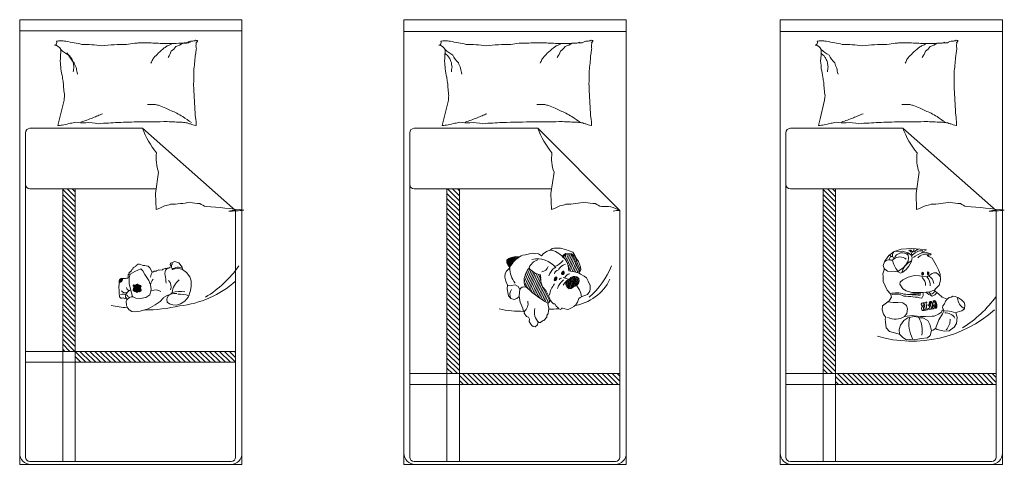
# Model space of a CAD drawing. Units: inches. Extents: x -17 to 1735, y -531 to 60.
# Tile 5 of 27: x 1734.6625 to 1734.8369, y -150.3996 to -150.3208. Entities that reach past the tile are written whole.
import ezdxf

# ---------------------------------------------------------------- set-up
doc = ezdxf.new("R2010")
doc.units = ezdxf.units.IN
doc.header["$MEASUREMENT"] = 0
doc.layers.add('A-FURN', color=242, linetype='Continuous', lineweight=18, true_color=0xcd2027)
pattern_1 = [(45, (81.6226725, 61.5392477), (-0.0019250982, 0.0019250982), [])]

# ---------------------------------------------------------------- blocks, each defined once
blk = doc.blocks.new('childrens_room_2')
h = blk.add_hatch()
h.set_pattern_fill('ANSI31', color=256, scale=0.005, style=0)
h.set_pattern_definition([(135, (71.032121, 52.193135), (0.01122532, 0.01122532), [])])
h.paths.add_polyline_path([(70.0407, 50.0124), (70.0966, 50.0124), (70.0966, 50.7433), (70.0407, 50.7433)])
h.paths.add_polyline_path([(70.0966, 49.9634), (70.8188, 49.9634), (70.8188, 50.0124), (70.0966, 50.0124)])
h = blk.add_hatch()
h.set_pattern_fill('ANSI31', color=256, scale=0.005, style=0)
h.set_pattern_definition([(135, (72.81088, 52.19314), (0.01122532, 0.01122532), [])])
h.paths.add_polyline_path([(71.8254, 49.9124), (71.8254, 50.7433), (71.7695, 50.7433), (71.7695, 49.9124)])
h.paths.add_polyline_path([(71.8254, 49.9124), (71.8254, 49.8634), (72.5475, 49.8634), (72.5475, 49.9124)])
h = blk.add_hatch()
h.set_pattern_fill('ANSI31', color=256, scale=0.005, style=0)
h.set_pattern_definition([(135, (74.453404, 52.19314), (0.01122532, 0.01122532), [])])
h.paths.add_polyline_path([(73.462, 49.9124), (73.5179, 49.9124), (73.5179, 50.7433), (73.462, 50.7433)])
h.paths.add_polyline_path([(73.5179, 49.9124), (73.5179, 49.8634), (74.2401, 49.8634), (74.2401, 49.9124)])
h = blk.add_hatch()
h.set_pattern_fill('ANSI31', color=256, scale=0.03, angle=22.8083, style=0)
h.set_pattern_definition([(67.808265, (80.8380315, 70.7464355), (-0.00347221906, 0.00141640207), [])])
h.paths.add_polyline_path([(72.0954, 50.4381), (72.0948, 50.4378), (72.0787, 50.4386), (72.0605, 50.4354), (72.0474, 50.4307), (72.0388, 50.4225), (72.0386, 50.4104), (72.043, 50.4018), (72.0493, 50.3939), (72.0525, 50.3899, -0.129501)])
h = blk.add_hatch()
h.set_pattern_fill('ANSI31', color=256, scale=0.06, angle=22.8083, style=0)
h.set_pattern_definition([(67.808265, (80.8380315, 70.7464355), (-0.006944438, 0.0028328041), [])])
h.paths.add_polyline_path([(72.3102, 50.4126), (72.3154, 50.3967), (72.3173, 50.3742), (72.3247, 50.3728), (72.3435, 50.3709), (72.3573, 50.367), (72.3611, 50.3828), (72.3527, 50.4011), (72.3398, 50.437), (72.3277, 50.4462), (72.3044, 50.4478), (72.2912, 50.4362), (72.3009, 50.4275)])
h.paths.add_polyline_path([(72.1906, 50.357, -0.19505), (72.1388, 50.3871, 0.242355), (72.1193, 50.3082, 0.070869), (72.2242, 50.2293), (72.2307, 50.2347), (72.2346, 50.2416), (72.226, 50.262), (72.2136, 50.2862), (72.1998, 50.3029), (72.1922, 50.3246)])
h = blk.add_hatch()
h.set_pattern_fill('ANSI31', color=256, scale=0.014175, angle=22.8083, style=0)
h.set_pattern_definition([(67.808265, (80.921218, 69.6912015), (-0.0016406235, 0.00066924998), [])])
h.paths.add_polyline_path([(72.2636, 50.3389), (72.2631, 50.3443), (72.261, 50.3472), (72.2563, 50.3444), (72.2535, 50.3405), (72.2519, 50.3331), (72.254, 50.3301), (72.2581, 50.3316), (72.2619, 50.3344)])
h.paths.add_polyline_path([(72.2967, 50.3631), (72.297, 50.3674), (72.2955, 50.3717), (72.2931, 50.3731), (72.2914, 50.373), (72.2889, 50.3705), (72.286, 50.3675), (72.2853, 50.3622), (72.2873, 50.3589), (72.2915, 50.3586)])
h = blk.add_hatch()
h.set_pattern_fill('ANSI31', color=256, scale=0.0042, style=0)
h.set_pattern_definition([(135, (58.9600481, 66.9732639), (0.00064315781, 0.00064315781), [])])
h.paths.add_polyline_path([(73.932, 50.3698), (73.9308, 50.3643), (73.9314, 50.3584), (73.9358, 50.3588), (73.9373, 50.3621), (73.937, 50.3676), (73.9355, 50.369)])
edge = h.paths.add_edge_path()
edge.add_line((73.907, 50.3689), (73.9051, 50.3646))
edge.add_line((73.9051, 50.3646), (73.9062, 50.3588))
edge.add_line((73.9062, 50.3588), (73.9091, 50.3556))
edge.add_line((73.9091, 50.3556), (73.9131, 50.3592))
edge.add_line((73.9131, 50.3592), (73.9127, 50.3649))
edge.add_line((73.9127, 50.3649), (73.9102, 50.3678))
edge.add_line((73.9102, 50.3678), (73.907, 50.3691))
h = blk.add_hatch()
h.set_pattern_fill('ANSI31', color=256, scale=0.02178, style=0)
h.set_pattern_definition(pattern_1)
h.paths.add_polyline_path([(70.3094, 50.3407), (70.3044, 50.3404), (70.3, 50.3387), (70.2967, 50.3345), (70.2953, 50.3312), (70.2944, 50.3226, 0.479357)])
h = blk.add_hatch()
h.set_pattern_fill('ANSI31', color=256, scale=0.035437, angle=22.8083, style=0)
h.set_pattern_definition([(67.808265, (80.921218, 69.6912015), (-0.0041015588, 0.0016731249), [])])
h.paths.add_polyline_path([(72.324, 50.34), (72.3114, 50.3334), (72.3076, 50.3302), (72.3049, 50.325), (72.3036, 50.3209), (72.3047, 50.3119), (72.3098, 50.3016), (72.319, 50.2933), (72.3275, 50.295), (72.3385, 50.3029), (72.3467, 50.3053), (72.353, 50.309), (72.3617, 50.3199), (72.3649, 50.3289), (72.362, 50.3398), (72.3538, 50.3477), (72.3447, 50.3499), (72.3375, 50.349), (72.3271, 50.3454)])
h = blk.add_hatch()
h.set_pattern_fill('ANSI31', color=256, scale=0.02178, style=0)
h.set_pattern_definition(pattern_1)
h.paths.add_polyline_path([(70.3802, 50.2814), (70.3856, 50.281), (70.3908, 50.2829), (70.3939, 50.2865), (70.3939, 50.2906), (70.3911, 50.2965), (70.3901, 50.3009), (70.3918, 50.303), (70.3932, 50.3057), (70.3918, 50.309), (70.3892, 50.3096), (70.3862, 50.3097), (70.3822, 50.3109), (70.3771, 50.3142), (70.3757, 50.3148), (70.3698, 50.3113), (70.3672, 50.3104), (70.363, 50.3111), (70.3601, 50.3115), (70.3574, 50.3089), (70.3584, 50.3061), (70.3611, 50.3038), (70.3606, 50.2987), (70.357, 50.2898), (70.3578, 50.2855), (70.3607, 50.2849), (70.3629, 50.2844), (70.3647, 50.2821), (70.3669, 50.2822), (70.3706, 50.281), (70.3732, 50.2785), (70.3746, 50.2772), (70.3762, 50.2793)])
for p, q in [((69.8472, 49.5044), (69.8472, 51.5044)), ((70.8472, 51.5044), (70.8472, 49.5044)), ((71.576, 49.5044), (71.576, 51.5044)), ((71.576, 51.5044), (72.576, 51.5044)), ((72.576, 51.5044), (72.576, 49.5044)), ((73.2685, 51.5044), (74.2685, 51.5044)), ((73.2685, 49.5044), (73.2685, 51.5044)), ((74.2685, 51.5044), (74.2685, 49.5044)), ((71.576, 51.452), (72.576, 51.452)), ((73.2685, 51.452), (74.2685, 51.452)), ((69.873, 50.9959), (69.873, 49.5366)), ((70.3998, 51.0159), (69.893, 51.0159)), ((70.3998, 51.0159), (70.8188, 50.6461)), ((71.6018, 50.9959), (71.6018, 49.5366)), ((72.1786, 51.0159), (71.6218, 51.0159)), ((72.1786, 51.0159), (72.5475, 50.6461)), ((73.2943, 50.9959), (73.2943, 49.5366)), ((73.8211, 51.0159), (73.3143, 51.0159)), ((73.8211, 51.0159), (74.2401, 50.6461)), ((69.893, 50.7433), (70.4616, 50.7433)), ((71.6218, 50.7433), (72.2404, 50.7433)), ((73.3143, 50.7433), (73.8829, 50.7433)), ((70.8188, 49.5366), (70.8188, 50.6461)), ((72.5475, 49.5366), (72.5475, 50.6461)), ((74.2401, 49.5366), (74.2401, 50.6461)), ((69.873, 50.0124), (70.8188, 50.0124)), ((69.873, 49.9634), (70.8188, 49.9634)), ((71.6018, 49.9124), (72.5475, 49.9124)), ((73.2943, 49.9124), (74.2401, 49.9124)), ((71.6018, 49.8634), (72.5475, 49.8634)), ((73.2943, 49.8634), (74.2401, 49.8634)), ((70.8472, 49.5044), (69.8472, 49.5044)), ((69.893, 49.5166), (70.7988, 49.5166)), ((72.576, 49.5044), (71.576, 49.5044)), ((71.6218, 49.5166), (72.5275, 49.5166)), ((73.2685, 49.5044), (74.2685, 49.5044)), ((73.3143, 49.5166), (74.2201, 49.5166))]:
    blk.add_line(p, q)
for points in [[(70.8472, 51.5044), (69.8472, 51.5044)], [(69.8472, 51.4544), (70.8472, 51.4544)], [(70.0407, 49.5166), (70.0407, 50.7433)], [(70.0966, 49.5166), (70.0966, 50.7433)], [(71.7695, 49.5166), (71.7695, 50.7433)], [(71.8254, 49.5166), (71.8254, 50.7433)], [(73.462, 49.5166), (73.462, 50.7433)], [(73.5179, 49.5166), (73.5179, 50.7433)], [(72.0525, 50.3899), (72.0483, 50.3837), (72.0371, 50.3729), (72.0308, 50.3628), (72.0297, 50.3457), (72.035, 50.3277), (72.0423, 50.3104), (72.0402, 50.2938), (72.0443, 50.2699), (72.0459, 50.2623), (72.0572, 50.2498), (72.0719, 50.2454), (72.0843, 50.2499), (72.0946, 50.2594), (72.0991, 50.2343), (72.1106, 50.2052), (72.1144, 50.1926), (72.1187, 50.1914), (72.1173, 50.184), (72.1272, 50.1693), (72.1357, 50.1669), (72.1407, 50.157), (72.1397, 50.1468), (72.1461, 50.1352), (72.1512, 50.1283), (72.1572, 50.1248), (72.1661, 50.1233), (72.1763, 50.1313), (72.1785, 50.1405), (72.1823, 50.1421), (72.1904, 50.1425), (72.1993, 50.15), (72.206, 50.1521), (72.2187, 50.1665), (72.2183, 50.1746), (72.2248, 50.1825), (72.2273, 50.2069), (72.2241, 50.2199), (72.2234, 50.2286), (72.2307, 50.2347), (72.2346, 50.2416), (72.2421, 50.2327), (72.2482, 50.227), (72.2544, 50.2266), (72.2614, 50.2153), (72.2676, 50.2096), (72.2725, 50.2034), (72.2797, 50.2004), (72.2839, 50.2029), (72.2843, 50.2076), (72.2898, 50.2069), (72.2995, 50.2035), (72.3131, 50.2016), (72.3181, 50.2022), (72.3291, 50.2084), (72.3403, 50.2138), (72.3492, 50.2213), (72.3572, 50.2345), (72.3624, 50.2509), (72.3689, 50.2552), (72.3805, 50.2616), (72.39, 50.2641), (72.4011, 50.268), (72.4124, 50.284), (72.4143, 50.2939), (72.4134, 50.3085), (72.4054, 50.3277), (72.3971, 50.3438), (72.3864, 50.3513), (72.3701, 50.3595), (72.3649, 50.3648), (72.3712, 50.3803), (72.3696, 50.3931), (72.3605, 50.4164), (72.3538, 50.4271), (72.345, 50.4445), (72.3353, 50.4585), (72.319, 50.4651), (72.3031, 50.4705), (72.2802, 50.4767), (72.2516, 50.4767), (72.2425, 50.4751), (72.234, 50.4685), (72.2209, 50.4638), (72.2031, 50.4525), (72.1946, 50.4422), (72.1816, 50.4517), (72.1683, 50.4529), (72.1647, 50.4507), (72.1522, 50.4537), (72.1225, 50.4472), (72.1108, 50.4446), (72.1032, 50.4429), (72.0987, 50.4395), (72.0948, 50.4378), (72.0787, 50.4386), (72.0605, 50.4354), (72.0474, 50.4307), (72.0388, 50.4225), (72.0386, 50.4104), (72.043, 50.4018), (72.0493, 50.3939), (72.0525, 50.3899)], [(73.9607, 50.287), (73.9801, 50.2714), (73.998, 50.2559), (74.0128, 50.2497), (74.0198, 50.2481), (74.0283, 50.2543), (74.0376, 50.2559), (74.0454, 50.2606), (74.0555, 50.259), (74.0703, 50.2528), (74.0843, 50.2443), (74.0967, 50.2318), (74.0998, 50.2217), (74.0983, 50.2039), (74.0858, 50.1945), (74.0641, 50.1883), (74.0586, 50.186), (74.0648, 50.1666), (74.0617, 50.1379), (74.0509, 50.1215), (74.0283, 50.1045), (74.0066, 50.1029), (73.9755, 50.1114), (73.9677, 50.1161), (73.9568, 50.1083), (73.9498, 50.1068), (73.9436, 50.0835), (73.9319, 50.0734), (73.9032, 50.0703), (73.8877, 50.068), (73.8706, 50.0641), (73.8519, 50.0656), (73.8371, 50.0648), (73.82, 50.0749), (73.8061, 50.0905), (73.7765, 50.0967), (73.7602, 50.1013), (73.7454, 50.1177), (73.7423, 50.1441), (73.7415, 50.1596), (73.7439, 50.165), (73.733, 50.1806), (73.7268, 50.1992), (73.7283, 50.2178), (73.7462, 50.2303), (73.7594, 50.2396), (73.7687, 50.2567), (73.7649, 50.2707), (73.7501, 50.2885), (73.7408, 50.3072), (73.7322, 50.3274), (73.7314, 50.3499), (73.7307, 50.3615), (73.7361, 50.3794), (73.7361, 50.3848), (73.7322, 50.3988), (73.7384, 50.4159), (73.7431, 50.4229), (73.7579, 50.4439), (73.7812, 50.4625), (73.813, 50.4726), (73.8605, 50.4757), (73.8978, 50.4726), (73.9273, 50.4695), (73.9164, 50.464), (73.9063, 50.4609), (73.9117, 50.4563), (73.925, 50.4578), (73.9483, 50.4516), (73.9444, 50.447), (73.9304, 50.4438), (73.9366, 50.4392), (73.9522, 50.4322), (73.9708, 50.3996), (73.9809, 50.3794), (73.9879, 50.3592), (73.9902, 50.3328), (73.984, 50.3103), (73.9708, 50.2963), (73.9607, 50.287)], [(73.7812, 50.4625), (73.8177, 50.4638), (73.8446, 50.4559), (73.8557, 50.4472), (73.8629, 50.4353), (73.8597, 50.4163), (73.847, 50.3957), (73.8359, 50.3815), (73.8201, 50.3688), (73.8106, 50.3641), (73.7995, 50.3704), (73.786, 50.3712), (73.7511, 50.3728), (73.7392, 50.3823), (73.7361, 50.3848)], [(73.7955, 50.3706), (73.8201, 50.3862), (73.8335, 50.4013), (73.8446, 50.4179), (73.8454, 50.433), (73.8446, 50.4456), (73.8415, 50.4543)], [(70.2942, 50.3148), (70.2935, 50.3015), (70.2945, 50.2859), (70.2951, 50.2694), (70.2957, 50.2645), (70.296, 50.2586), (70.3026, 50.2523), (70.3088, 50.252), (70.3134, 50.2533), (70.3181, 50.2502), (70.3225, 50.2514), (70.3306, 50.248), (70.3299, 50.2439), (70.3268, 50.2383), (70.3274, 50.2184), (70.3334, 50.2069), (70.3396, 50.1998), (70.3517, 50.192), (70.3645, 50.1901), (70.3894, 50.1929), (70.4245, 50.2044), (70.456, 50.2219), (70.4796, 50.2365), (70.4924, 50.2517), (70.4949, 50.2551), (70.5135, 50.2648), (70.5154, 50.2651), (70.5173, 50.2632), (70.5111, 50.2539), (70.5092, 50.247), (70.5107, 50.2337), (70.5213, 50.2265), (70.5358, 50.2218), (70.5533, 50.2211), (70.5708, 50.2258), (70.5903, 50.2386), (70.6057, 50.2568), (70.6098, 50.2675), (70.6105, 50.2736), (70.6158, 50.287), (70.6185, 50.3052), (70.6185, 50.3294), (70.6131, 50.3482), (70.5983, 50.367), (70.5802, 50.3811), (70.5782, 50.3906), (70.5634, 50.4114), (70.5452, 50.4161), (70.5257, 50.4087), (70.5243, 50.402), (70.53, 50.3953), (70.5305, 50.3934), (70.524, 50.3907), (70.5196, 50.3885), (70.5185, 50.3874), (70.5127, 50.3863), (70.5108, 50.3849), (70.5015, 50.386), (70.4927, 50.3816), (70.4899, 50.3786), (70.4782, 50.3783), (70.4729, 50.3797), (70.4628, 50.3753), (70.4617, 50.3734), (70.4524, 50.3726), (70.4458, 50.3687), (70.4414, 50.3709), (70.4381, 50.3775), (70.4329, 50.3879), (70.4247, 50.3951), (70.4159, 50.3972), (70.4109, 50.3989), (70.4033, 50.3994), (70.3975, 50.4005), (70.3906, 50.4038), (70.3868, 50.4052), (70.3799, 50.4049), (70.3714, 50.3981), (70.3703, 50.3942), (70.3627, 50.3909), (70.3583, 50.3879), (70.3569, 50.3841), (70.3547, 50.3822), (70.3522, 50.3805), (70.3495, 50.3748), (70.3484, 50.3734), (70.3465, 50.3734), (70.3413, 50.3679), (70.3388, 50.3654), (70.3391, 50.3611), (70.3355, 50.3567), (70.3358, 50.3528), (70.3352, 50.3457), (70.3344, 50.3424), (70.3336, 50.3411), (70.332, 50.3416), (70.3272, 50.342), (70.3236, 50.3402), (70.3216, 50.34), (70.3128, 50.3409), (70.3044, 50.3404), (70.3, 50.3387), (70.2967, 50.3345), (70.2953, 50.3312), (70.294, 50.3185), (70.2942, 50.3148)], [(72.2876, 50.4403), (72.3025, 50.4534), (72.3297, 50.4516), (72.3444, 50.4404), (72.3578, 50.4032), (72.3669, 50.3834), (72.3627, 50.3657)], [(72.2912, 50.4362), (72.3044, 50.4478), (72.3277, 50.4462), (72.3398, 50.437), (72.3527, 50.4011), (72.3611, 50.3828), (72.3573, 50.367)], [(72.3649, 50.3648), (72.3435, 50.3709), (72.3247, 50.3728), (72.3173, 50.3742), (72.3154, 50.3967), (72.3102, 50.4126), (72.3009, 50.4275), (72.2912, 50.4362)], [(70.3435, 50.3603), (70.3654, 50.3725), (70.3925, 50.3839), (70.4013, 50.3747), (70.4109, 50.3589), (70.4284, 50.3314), (70.4363, 50.3117), (70.4385, 50.2907), (70.4323, 50.2662), (70.4144, 50.2549), (70.3886, 50.25), (70.3693, 50.2522), (70.3553, 50.2601), (70.3457, 50.2925), (70.34, 50.3183), (70.3391, 50.3454), (70.3435, 50.3603)], [(72.286, 50.3675), (72.2853, 50.3622), (72.2873, 50.3589), (72.2915, 50.3586), (72.2967, 50.3631), (72.297, 50.3674), (72.2955, 50.3717), (72.2931, 50.3731), (72.2914, 50.373), (72.2889, 50.3705), (72.286, 50.3675)], [(73.907, 50.3689), (73.9051, 50.3646), (73.9062, 50.3588), (73.9091, 50.3556), (73.9131, 50.3592), (73.9127, 50.3649), (73.9102, 50.3678), (73.907, 50.3691)], [(73.9281, 50.3476), (73.9427, 50.3574), (73.9517, 50.3629), (73.9592, 50.366), (73.9718, 50.366), (73.9804, 50.359), (73.9891, 50.346)], [(73.932, 50.3698), (73.9308, 50.3643), (73.9314, 50.3584), (73.9358, 50.3588), (73.9373, 50.3621), (73.937, 50.3676), (73.9355, 50.369), (73.932, 50.3698)], [(72.1906, 50.357), (72.1922, 50.3246), (72.1998, 50.3029), (72.2136, 50.2862), (72.226, 50.262), (72.2346, 50.2416)], [(72.2535, 50.3405), (72.2519, 50.3331), (72.254, 50.3301), (72.2581, 50.3316), (72.2619, 50.3344), (72.2636, 50.3389), (72.2631, 50.3443), (72.261, 50.3472), (72.2563, 50.3444), (72.2535, 50.3405)], [(72.324, 50.34), (72.3114, 50.3334), (72.3076, 50.3302), (72.3049, 50.325), (72.3036, 50.3209), (72.3047, 50.3119), (72.3098, 50.3016), (72.319, 50.2933), (72.3275, 50.295), (72.3385, 50.3029), (72.3467, 50.3053), (72.353, 50.309), (72.3617, 50.3199), (72.3649, 50.3289), (72.362, 50.3398), (72.3538, 50.3477), (72.3447, 50.3499), (72.3375, 50.349), (72.3271, 50.3454), (72.324, 50.34)], [(73.9281, 50.3476), (73.9097, 50.3487), (73.8955, 50.3527), (73.8727, 50.3542), (73.8437, 50.3468), (73.8197, 50.3342), (73.8091, 50.3232), (73.8067, 50.3142), (73.8205, 50.2946), (73.835, 50.2843), (73.861, 50.2773), (73.9085, 50.2769), (73.9411, 50.28), (73.9521, 50.2847), (73.9607, 50.287)], [(70.3757, 50.3148), (70.3698, 50.3113), (70.3672, 50.3104), (70.363, 50.3111), (70.3601, 50.3115), (70.3574, 50.3089), (70.3584, 50.3061), (70.3611, 50.3038), (70.3606, 50.2987), (70.357, 50.2898), (70.3578, 50.2855), (70.3607, 50.2849), (70.3629, 50.2844), (70.3647, 50.2821), (70.3669, 50.2822), (70.3706, 50.281), (70.3732, 50.2785), (70.3746, 50.2772), (70.3762, 50.2793), (70.3802, 50.2814), (70.3856, 50.281), (70.3908, 50.2829), (70.3939, 50.2865), (70.3939, 50.2906), (70.3911, 50.2965), (70.3901, 50.3009), (70.3918, 50.303), (70.3932, 50.3057), (70.3918, 50.309), (70.3892, 50.3096), (70.3862, 50.3097), (70.3822, 50.3109), (70.3771, 50.3142), (70.3757, 50.3148)], [(72.0423, 50.3104), (72.0593, 50.3093), (72.076, 50.3126), (72.0898, 50.3048), (72.097, 50.2913), (72.0953, 50.2793), (72.0946, 50.2594)], [(73.7528, 50.2349), (73.777, 50.2325), (73.7977, 50.2321), (73.8201, 50.2304), (73.8362, 50.2185), (73.8417, 50.2037), (73.8383, 50.1822), (73.8281, 50.1691), (73.8404, 50.1708), (73.8637, 50.1737)], [(73.9258, 50.2304), (73.9279, 50.2322), (73.9278, 50.2337), (73.924, 50.2335), (73.9098, 50.2315), (73.9051, 50.2296), (73.903, 50.2251), (73.9037, 50.2201), (73.9067, 50.2168), (73.9101, 50.2155), (73.908, 50.2132), (73.9055, 50.2113), (73.9039, 50.2075), (73.9056, 50.2001), (73.9095, 50.1971), (73.9169, 50.1971), (73.9315, 50.1991), (73.932, 50.201), (73.9288, 50.2016), (73.9258, 50.2304)], [(73.9401, 50.2223), (73.9335, 50.2223), (73.9322, 50.2205), (73.9355, 50.2198), (73.9381, 50.2139), (73.9408, 50.2111), (73.9396, 50.2071), (73.936, 50.2061), (73.934, 50.2068), (73.9358, 50.2025), (73.9393, 50.2003), (73.9444, 50.2018), (73.9464, 50.2035), (73.9482, 50.2035), (73.9515, 50.2023), (73.9568, 50.2033), (73.9606, 50.2081), (73.9599, 50.2152), (73.9568, 50.2205), (73.9535, 50.2228), (73.9538, 50.2289), (73.9515, 50.2342), (73.9477, 50.2372), (73.9439, 50.2372), (73.9398, 50.2344), (73.9391, 50.2301), (73.9416, 50.2253), (73.9462, 50.2228), (73.9434, 50.2142), (73.9424, 50.2127), (73.9398, 50.2165), (73.9393, 50.22), (73.9411, 50.2215), (73.9401, 50.2223)], [(73.9452, 50.2342), (73.9439, 50.2309), (73.9454, 50.2271), (73.9469, 50.2266), (73.9479, 50.2301), (73.9472, 50.2334), (73.9459, 50.2342), (73.9452, 50.2342)], [(73.9593, 50.2296), (73.9581, 50.2357), (73.9566, 50.2403), (73.9586, 50.2393), (73.9604, 50.2405), (73.9626, 50.241), (73.9687, 50.2362), (73.9733, 50.2236), (73.9735, 50.2111), (73.972, 50.2071), (73.9685, 50.2063), (73.9624, 50.2071), (73.9609, 50.2162), (73.9601, 50.2198), (73.9606, 50.2215), (73.9672, 50.2223), (73.969, 50.2215), (73.9664, 50.218), (73.9672, 50.2101), (73.9697, 50.2089), (73.9707, 50.2124), (73.9697, 50.22), (73.968, 50.2273), (73.9654, 50.2362), (73.9631, 50.2372), (73.9606, 50.2334), (73.9606, 50.2294), (73.9593, 50.2294), (73.9593, 50.2296)], [(74.0198, 50.2481), (74.0126, 50.2384), (74.008, 50.2262), (74.0004, 50.2169), (73.9991, 50.208), (74.0054, 50.1978)], [(73.9978, 50.1983), (73.9949, 50.1894), (73.9813, 50.1796), (73.9606, 50.1703), (73.9525, 50.1708), (73.9225, 50.1695), (73.8992, 50.1695), (73.8717, 50.172), (73.8637, 50.1737)], [(73.9169, 50.2298), (73.9192, 50.2176), (73.9158, 50.2172), (73.9132, 50.2193), (73.9122, 50.2254), (73.9135, 50.2293), (73.9168, 50.2299)], [(73.9196, 50.2147), (73.921, 50.2004), (73.9196, 50.1997), (73.9153, 50.2006), (73.9137, 50.2028), (73.9132, 50.2093), (73.915, 50.214), (73.9171, 50.2151), (73.9196, 50.2147)], [(73.9528, 50.2195), (73.949, 50.2084), (73.9482, 50.2071), (73.9512, 50.2063), (73.954, 50.2106), (73.9545, 50.219), (73.9528, 50.2196)], [(73.9677, 50.1161), (73.9817, 50.1543), (73.9987, 50.1818), (74.0054, 50.1928)], [(74.0054, 50.1928), (74.0054, 50.1978), (73.9978, 50.1983)], [(74.0586, 50.186), (74.0384, 50.1915), (74.0211, 50.1953), (74.0054, 50.1928)], [(73.8061, 50.0905), (73.8045, 50.1103), (73.8095, 50.1298), (73.8243, 50.1517), (73.8434, 50.1627), (73.8569, 50.167), (73.8717, 50.1687), (73.8891, 50.1657), (73.8963, 50.1627), (73.9098, 50.1632), (73.9327, 50.1509), (73.9415, 50.1336), (73.9498, 50.1068)]]:
    blk.add_lwpolyline(points)
for points in [[(70.0323, 51.3708, 0.263368), (70.0043, 51.3896, 0.494818), (70.0135, 51.4083, 0.049225), (70.0312, 51.4101, 0.036831), (70.0548, 51.4083, 0.031893), (70.0928, 51.4002, -0.035782), (70.1267, 51.3932, -0.032941), (70.2164, 51.3873, -0.026564), (70.3276, 51.3932, -0.017905), (70.3651, 51.3986, 0.033397), (70.3853, 51.4008, 0.03204), (70.4224, 51.4001, -0.018442), (70.4867, 51.3971, -0.010837), (70.5515, 51.3978, -0.014624), (70.5994, 51.4008, -0.111249), (70.6219, 51.4081, 0.153708), (70.6388, 51.4121, 0.076444), (70.6463, 51.4104, 0.215512), (70.6482, 51.4083, 0.585858), (70.6456, 51.4053, -0.363489), (70.6407, 51.4027, -0.191716), (70.6406, 51.3912, 0.129675), (70.6426, 51.3745, 0.01735), (70.6396, 51.3577, -0.019326), (70.6369, 51.3426, -0.018818), (70.6303, 51.2743, -0.021828), (70.6294, 51.215, -0.006204), (70.6308, 51.1812, -0.001963), (70.6369, 51.0743, -0.028341), (70.6412, 51.0382, 0.117014), (70.6407, 51.0293, 0.36606), (70.6393, 51.0283, 0.03973), (70.6257, 51.0311, 0.048309), (70.6119, 51.0366, -0.062981), (70.6013, 51.0405, -0.04058), (70.5779, 51.0439, -0.014345), (70.5111, 51.0461, -0.005484), (70.3857, 51.0454, -0.007153), (70.2895, 51.0424, -0.008762), (70.247, 51.0397, 0.008153), (70.2013, 51.0368, 0.06251), (70.1442, 51.0412, -0.078669), (70.0986, 51.0432, -0.047825), (70.0762, 51.0385, 0.034494), (70.0454, 51.0311, 0.023571), (70.0201, 51.0281, 0.510228), (70.0191, 51.0293), (70.0266, 51.0593), (70.0473, 51.1419, -0.073041), (70.0493, 51.1614, -0.023305), (70.0435, 51.2225, -0.018299), (70.0395, 51.2454, 0.01097), (70.0321, 51.2834, 0.042281), (70.0292, 51.3177, 0.027201), (70.0321, 51.3711)], [(70.5341, 51.397, -0.027842), (70.5103, 51.3864, -0.048685), (70.4978, 51.3783, -0.023666), (70.4699, 51.3539, -0.031223), (70.4508, 51.3333, -0.046801), (70.4457, 51.3256, -0.023191), (70.4377, 51.3089)], [(70.6161, 51.4027, -0.088153), (70.5816, 51.3992, -0.088153), (70.5504, 51.3839, -0.077547), (70.5287, 51.3623, -0.077547), (70.5147, 51.3351)], [(71.761, 51.3708, 0.263368), (71.7331, 51.3896, 0.494818), (71.7423, 51.4083, 0.049225), (71.7599, 51.4101, 0.036831), (71.7836, 51.4083, 0.031893), (71.8215, 51.4002, -0.035782), (71.8555, 51.3932, -0.032941), (71.9451, 51.3873, -0.026564), (72.0564, 51.3932, -0.017905), (72.0939, 51.3986, 0.009667), (72.1641, 51.4008, 0.03204), (72.2012, 51.4001, -0.018442), (72.2655, 51.3971, -0.010837), (72.3302, 51.3978, -0.014624), (72.3781, 51.4008, -0.111249), (72.4007, 51.4081, 0.153708), (72.4176, 51.4121, 0.076444), (72.425, 51.4104, 0.215512), (72.427, 51.4083, 0.585858), (72.4243, 51.4053, -0.363489), (72.4195, 51.4027, -0.191716), (72.4194, 51.3912, 0.129675), (72.4213, 51.3746, 0.01735), (72.4183, 51.3577, -0.019326), (72.4157, 51.3427, -0.018818), (72.4091, 51.2743, -0.021828), (72.4082, 51.215, -0.006204), (72.4096, 51.1812, -0.001963), (72.4157, 51.0743, -0.028341), (72.42, 51.0382, 0.117014), (72.4195, 51.0293, 0.36606), (72.418, 51.0283, 0.03973), (72.4044, 51.0311, 0.048309), (72.3907, 51.0366, -0.062981), (72.38, 51.0405, -0.04058), (72.3566, 51.0439, -0.014345), (72.2899, 51.0461, -0.005484), (72.1644, 51.0454, -0.004707), (72.0183, 51.0424, -0.008762), (71.9758, 51.0397, 0.008153), (71.93, 51.0368, 0.06251), (71.8729, 51.0412, -0.078669), (71.8273, 51.0432, -0.047825), (71.805, 51.0385, 0.034494), (71.7742, 51.0311, 0.023571), (71.7488, 51.0281, 0.510228), (71.7479, 51.0293), (71.7554, 51.0593), (71.7761, 51.1419, -0.073041), (71.778, 51.1614, -0.023305), (71.7723, 51.2225, -0.018299), (71.7682, 51.2454, 0.01097), (71.7609, 51.2834, 0.042281), (71.758, 51.3177, 0.027201), (71.7609, 51.3711)], [(72.2849, 51.397, -0.027842), (72.2611, 51.3864, -0.048685), (72.2486, 51.3783, -0.023666), (72.2207, 51.3539, -0.031223), (72.2016, 51.3333, -0.046801), (72.1965, 51.3256, -0.023191), (72.1885, 51.3089)], [(72.3669, 51.4027, -0.088153), (72.3324, 51.3992, -0.088153), (72.3012, 51.3839, -0.077547), (72.2795, 51.3623, -0.077547), (72.2655, 51.3351)], [(73.4536, 51.3708, 0.263368), (73.4256, 51.3896, 0.494818), (73.4348, 51.4083, 0.049225), (73.4525, 51.4101, 0.036831), (73.4761, 51.4083, 0.031893), (73.5141, 51.4002, -0.035782), (73.548, 51.3932, -0.032941), (73.6376, 51.3873, -0.026564), (73.7489, 51.3932, -0.017905), (73.7864, 51.3986, 0.033397), (73.8066, 51.4008, 0.03204), (73.8437, 51.4001, -0.018442), (73.908, 51.3971, -0.010837), (73.9728, 51.3978, -0.014624), (74.0207, 51.4008, -0.111249), (74.0432, 51.4081, 0.153708), (74.0601, 51.4121, 0.076444), (74.0675, 51.4104, 0.215512), (74.0695, 51.4083, 0.585858), (74.0668, 51.4053, -0.363489), (74.062, 51.4027, -0.191716), (74.0619, 51.3912, 0.129675), (74.0639, 51.3746, 0.01735), (74.0609, 51.3577, -0.019326), (74.0582, 51.3427, -0.018818), (74.0516, 51.2743, -0.021828), (74.0507, 51.215, -0.006204), (74.0521, 51.1812, -0.001963), (74.0582, 51.0743, -0.028341), (74.0625, 51.0382, 0.117014), (74.062, 51.0293, 0.36606), (74.0606, 51.0283, 0.03973), (74.047, 51.0311, 0.048309), (74.0332, 51.0366, -0.062981), (74.0226, 51.0405, -0.04058), (73.9992, 51.0439, -0.014345), (73.9324, 51.0461, -0.005484), (73.807, 51.0454, -0.007153), (73.7108, 51.0424, -0.008762), (73.6683, 51.0397, 0.008153), (73.6226, 51.0368, 0.06251), (73.5654, 51.0412, -0.078669), (73.5199, 51.0432, -0.047825), (73.4975, 51.0385, 0.034494), (73.4667, 51.0311, 0.023571), (73.4414, 51.0281, 0.510228), (73.4404, 51.0293), (73.4479, 51.0593), (73.4686, 51.1419, -0.073041), (73.4705, 51.1614, -0.023305), (73.4648, 51.2225, -0.018299), (73.4608, 51.2454, 0.01097), (73.4534, 51.2834, 0.042281), (73.4505, 51.3177, 0.027201), (73.4534, 51.3711)], [(73.9274, 51.397, -0.027842), (73.9036, 51.3864, -0.048685), (73.8911, 51.3783, -0.023666), (73.8632, 51.3539, -0.031223), (73.8442, 51.3333, -0.046801), (73.839, 51.3256, -0.023191), (73.831, 51.3089)], [(74.0094, 51.4027, -0.088153), (73.9749, 51.3992, -0.088153), (73.9437, 51.3839, -0.077547), (73.922, 51.3623, -0.077547), (73.908, 51.3351)], [(70.0321, 51.3708, 0.077379), (70.0669, 51.3455, 0.077379), (70.0924, 51.3107, 0.047525), (70.1023, 51.2861, 0.047525), (70.1074, 51.2601)], [(70.0586, 51.3548, 0.05369), (70.0728, 51.3418, 0.070312), (70.0809, 51.3295, 0.015448), (70.0846, 51.321, 0.013244), (70.0884, 51.3107, 0.082127), (70.0914, 51.2927, 0.064164), (70.0884, 51.2695)], [(71.7594, 51.3548, 0.05369), (71.7736, 51.3418, 0.070312), (71.7817, 51.3295, 0.015448), (71.7854, 51.321, 0.013244), (71.7892, 51.3107, 0.082127), (71.7922, 51.2927, 0.064164), (71.7892, 51.2695)], [(71.7609, 51.3708, 0.077379), (71.7957, 51.3455, 0.077379), (71.8211, 51.3107, 0.047525), (71.8311, 51.2861, 0.047525), (71.8361, 51.2601)], [(73.4519, 51.3548, 0.05369), (73.4661, 51.3418, 0.070312), (73.4742, 51.3295, 0.015448), (73.478, 51.321, 0.013244), (73.4817, 51.3107, 0.082127), (73.4847, 51.2927, 0.064164), (73.4817, 51.2695)], [(73.4534, 51.3708, 0.077379), (73.4882, 51.3455, 0.077379), (73.5137, 51.3107, 0.047525), (73.5236, 51.2861, 0.047525), (73.5287, 51.2601)], [(70.6198, 51.0424, -0.016108), (70.5809, 51.0686, -0.024599), (70.5541, 51.0837, -0.009477), (70.5051, 51.107, -0.015937), (70.4752, 51.1193, -0.072521), (70.4589, 51.1229, -0.033339), (70.4227, 51.1231)], [(72.3706, 51.0424, -0.016108), (72.3317, 51.0686, -0.024599), (72.3049, 51.0837, -0.009477), (72.2559, 51.107, -0.015937), (72.226, 51.1193, -0.072521), (72.2097, 51.1229, -0.033339), (72.1735, 51.1231)], [(74.0132, 51.0424, -0.016108), (73.9742, 51.0686, -0.024599), (73.9474, 51.0837, -0.009477), (73.8984, 51.107, -0.015937), (73.8686, 51.1193, -0.072521), (73.8522, 51.1229, -0.033339), (73.816, 51.1231)], [(70.1227, 51.0439, -0.009729), (70.15, 51.0529, -0.009729), (70.1769, 51.063, -0.007971), (70.1986, 51.0721, -0.007971), (70.2201, 51.0818)], [(71.8514, 51.0439, -0.009729), (71.8787, 51.053, -0.009729), (71.9056, 51.063, -0.007971), (71.9274, 51.0721, -0.007971), (71.9488, 51.0818)], [(73.5439, 51.0439, -0.009729), (73.5712, 51.053, -0.009729), (73.5982, 51.063, -0.007971), (73.6199, 51.0721, -0.007971), (73.6413, 51.0818)], [(70.3998, 51.0159, 0.085272), (70.4631, 50.9058, 0.124044), (70.4723, 50.8182), (70.4587, 50.7228), (70.4605, 50.6503)], [(72.1786, 51.0159, 0.085272), (72.2419, 50.9058, 0.124044), (72.2511, 50.8182), (72.2375, 50.7228), (72.2392, 50.6503)], [(73.8211, 51.0159, 0.085272), (73.8844, 50.9058, 0.124044), (73.8936, 50.8182), (73.88, 50.7228), (73.8817, 50.6503)], [(70.4605, 50.6503, 0.027362), (70.499, 50.6667, 0.040834), (70.5261, 50.6741, 0.038441), (70.6138, 50.6836, 0.076528), (70.6579, 50.6783, 0.103649), (70.6854, 50.6639, -0.018778), (70.8556, 50.6474, -0.024037), (70.7877, 50.6436, -0.052315), (70.8188, 50.6461)], [(73.8817, 50.6503, 0.027362), (73.9203, 50.6667, 0.040834), (73.9474, 50.6741, 0.038441), (74.0351, 50.6837, 0.076528), (74.0792, 50.6783, 0.103649), (74.1067, 50.6639, -0.018778), (74.2769, 50.6474, -0.024037), (74.209, 50.6436, -0.052315), (74.2401, 50.6461)]]:
    blk.add_lwpolyline(points, format="xyb")
for centre, radius, start, end in [((69.893, 50.9959), 0.02, 90, 180), ((71.6218, 50.9959), 0.02, 90, 180), ((73.3143, 50.9959), 0.02, 90, 180), ((69.893, 50.7633), 0.02, 180, 270), ((71.6218, 50.7633), 0.02, 180, 270), ((73.3143, 50.7633), 0.02, 180, 270), ((72.287, 51.248), 0.5741, 271.7887, 280.5945), ((72.4321, 50.8243), 0.1461, 254.2839, 271.7887), ((72.4847, 50.7367), 0.0757, 230.6139, 254.2839), ((72.1084, 51.0106), 0.3833, 289.9478, 296.2172), ((72.2461, 50.8362), 0.1724, 280.5945, 289.9478), ((72.4807, 50.5374), 0.1276, 58.4201, 97.4443), ((72.5439, 50.4969), 0.1493, 88.5957, 100.5745), ((72.2193, 50.3757), 0.094, 40.0646, 81.0184), ((73.8032, 50.4436), 0.0293, 143.5765, 191.2279), ((73.8179, 50.4187), 0.0374, 43.8678, 162.0903), ((73.8401, 50.4476), 0.021, 359.8396, 76.0806), ((73.8487, 50.4541), 0.0152, 13.2274, 78.5197), ((73.9097, 50.4021), 0.0638, 89.6164, 142.1678), ((73.858, 50.4685), 0.0116, 313.574, 16.7547), ((73.947, 50.3363), 0.1261, 109.0207, 128.9686), ((73.888, 50.4509), 0.0182, 87.0079, 149.847), ((72.1653, 50.3326), 0.1265, 119.3586, 153.0552), ((72.1927, 50.369), 0.0568, 104.7325, 161.4551), ((72.1767, 50.3269), 0.1025, 36.6141, 103.9334), ((72.2313, 50.4679), 0.0765, 287.6284, 321.9822), ((73.763, 50.3866), 0.0381, 90.7819, 130.2689), ((73.7701, 50.4298), 0.00919, 344.764, 214.1376), ((73.7739, 50.4494), 0.0122, 190.8913, 244.4656), ((73.7694, 50.4336), 0.0114, 232.183, 326.7186), ((73.8814, 50.4436), 0.1092, 190.7154, 219.1959), ((73.807, 50.3914), 0.0457, 50.6951, 127.9261), ((73.8951, 50.3471), 0.0814, 115.8144, 166.2159), ((73.9297, 50.3881), 0.0622, 81.4345, 132.5573), ((70.5819, 50.3063), 0.1522, 155.3415, 164.4913), ((70.5274, 50.363), 0.0275, 127.108, 198.2435), ((70.52, 50.3822), 0.0132, 353.9542, 51.018), ((70.5452, 50.3949), 0.016, 128.3031, 168.9374), ((70.5597, 50.3506), 0.0403, 61.149, 131.3836), ((70.5571, 50.3167), 0.0685, 70.3319, 110.5181), ((70.4067, 50.7031), 0.5256, 301.7708, 324.3375), ((72.1497, 50.3842), 0.0974, 176.6283, 221.5254), ((72.2056, 50.3287), 0.0888, 138.8697, 193.3627), ((72.2018, 50.4359), 0.0797, 217.7547, 261.9024), ((72.1933, 50.4022), 0.0317, 275.5542, 345.9589), ((72.3305, 50.3065), 0.1131, 133.4778, 156.0857), ((72.2711, 50.3595), 0.0186, 94.2478, 176.558), ((72.3115, 50.3589), 0.0461, 101.014, 151.9838), ((72.1653, 50.5364), 0.3715, 311.0314, 337.8934), ((70.2947, 50.3377), 0.015, 269.0987, 11.5429), ((70.4771, 50.3094), 0.0408, 136.7949, 176.7156), ((70.3713, 50.3208), 0.1343, 359.2848, 14.5089), ((70.4913, 50.3039), 0.0373, 337.4286, 46.0363), ((70.6109, 50.2709), 0.0777, 125.9219, 175.4055), ((70.5242, 50.6549), 0.4393, 275.4641, 312.1092), ((72.333, 50.2772), 0.0687, 124.8006, 164.2713), ((72.2851, 50.3312), 0.011, 90.1097, 167.3601), ((72.2719, 50.2434), 0.1039, 8.3054, 78.9473), ((72.5886, 50.1062), 0.3593, 141.9927, 145.4886), ((72.333, 50.324), 0.0393, 106.6236, 147.032), ((72.3234, 50.3151), 0.0146, 274.9536, 77.0589), ((72.3303, 50.3222), 0.0177, 7.7782, 95.1837), ((72.3363, 50.3185), 0.013, 280.7395, 28.1073), ((72.3056, 50.435), 0.2204, 279.4371, 333.5432), ((72.3454, 50.334), 0.00965, 284.3938, 14.927), ((73.8776, 50.3106), 0.0451, 358.5819, 49.3705), ((73.8937, 50.3123), 0.0493, 353.4892, 45.7022), ((73.9185, 50.3149), 0.0412, 4.4845, 65.7537), ((70.3263, 50.3031), 0.0276, 219.7451, 271.7337), ((70.3653, 50.2495), 0.0443, 120.5886, 163.4912), ((70.3488, 50.3039), 0.0216, 189.9605, 241.843), ((70.4598, 50.2463), 0.0426, 57.515, 117.2356), ((70.4983, 50.3058), 0.0453, 293.4063, 320.8909), ((70.568, 50.1443), 0.1372, 81.0084, 104.554), ((72.0924, 50.2681), 0.0397, 144.8325, 207.5513), ((72.1165, 50.2802), 0.0225, 73.0797, 150.2757), ((72.4486, 50.6372), 0.4656, 224.9707, 241.1855), ((72.3342, 50.2481), 0.1054, 140.1138, 170.2426), ((73.9084, 50.2716), 0.0161, 160.2357, 181.2203), ((73.9324, 50.2712), 0.0346, 170.4378, 189.1158), ((73.8846, 50.2694), 0.0274, 321.1866, 17.3611), ((74.009, 50.3853), 0.1368, 231.1517, 245.393), ((73.9521, 50.2832), 0.0141, 194.1166, 243.8166), ((73.9473, 50.2871), 0.0166, 264.9584, 350.1101), ((70.3138, 50.2277), 0.0427, 74.8422, 107.2397), ((70.3354, 50.2612), 0.0126, 176.1994, 229.0666), ((70.3466, 50.2734), 0.0186, 205.2148, 249.8011), ((70.3574, 50.2255), 0.0331, 92.1498, 146.1783), ((70.5462, 50.2018), 0.0709, 82.9692, 106.7988), ((70.5673, 50.1635), 0.1066, 67.6837, 94.5902), ((72.0901, 50.2272), 0.0441, 306.8303, 14.4951), ((73.7914, 50.1778), 0.098, 69.9535, 106.3269), ((73.7919, 50.21), 0.0606, 56.2013, 114.8632), ((73.9289, 51.4661), 1.2007, 265.0385, 268.5505), ((73.8232, 49.8355), 0.4249, 78.758, 89.6728), ((73.8762, 50.0967), 0.1752, 84.7212, 101.3428), ((73.9424, 50.2967), 0.0371, 285.0951, 327.2605), ((74.1207, 50.2543), 0.0543, 181.7111, 245.4409), ((73.8128, 50.566), 0.5256, 301.7708, 324.3375), ((70.4398, 51.2049), 1.0025, 259.6217, 263.7472), ((70.4093, 50.8574), 0.6588, 269.7962, 283.7616), ((72.114, 50.7553), 0.5627, 258.8153, 270.0463), ((72.2301, 50.1897), 0.0675, 166.5554, 224.9062), ((72.2189, 51.2049), 1.0025, 270.4734, 273.0628), ((73.8613, 50.6199), 0.5613, 253.9682, 311.5222), ((73.7866, 50.2379), 0.0803, 244.5538, 301.1116), ((73.9948, 50.1378), 0.1472, 169.3969, 207.7251), ((73.7933, 50.1082), 0.1141, 348.6714, 29.4122), ((74.0129, 50.1383), 0.0478, 29.5054, 94.8769), ((73.9676, 50.1549), 0.0658, 316.2853, 2.0233), ((69.8972, 49.5544), 0.05, 180, 270), ((69.893, 49.5366), 0.02, 180, 270), ((70.7972, 49.5544), 0.05, 270, 0), ((70.7988, 49.5366), 0.02, 270, 0), ((71.626, 49.5544), 0.05, 180, 270), ((71.6218, 49.5366), 0.02, 180, 270), ((72.526, 49.5544), 0.05, 270, 0), ((72.5275, 49.5366), 0.02, 270, 0), ((73.3185, 49.5544), 0.05, 180, 270), ((73.3143, 49.5366), 0.02, 180, 270), ((74.2185, 49.5544), 0.05, 270, 0), ((74.2201, 49.5366), 0.02, 270, 0)]:
    blk.add_arc(centre, radius, start, end)

msp = doc.modelspace()

# ---------------------------------------------------------------- block references
at = {"layer": 'A-FURN', "xscale": 0.0393700787401575, "yscale": 0.0393700787401575, "zscale": 0.0393700787401575}
msp.add_blockref('childrens_room_2', (1731.9126, -152.34857), dxfattribs=at)

doc.saveas('drawing.dxf')
